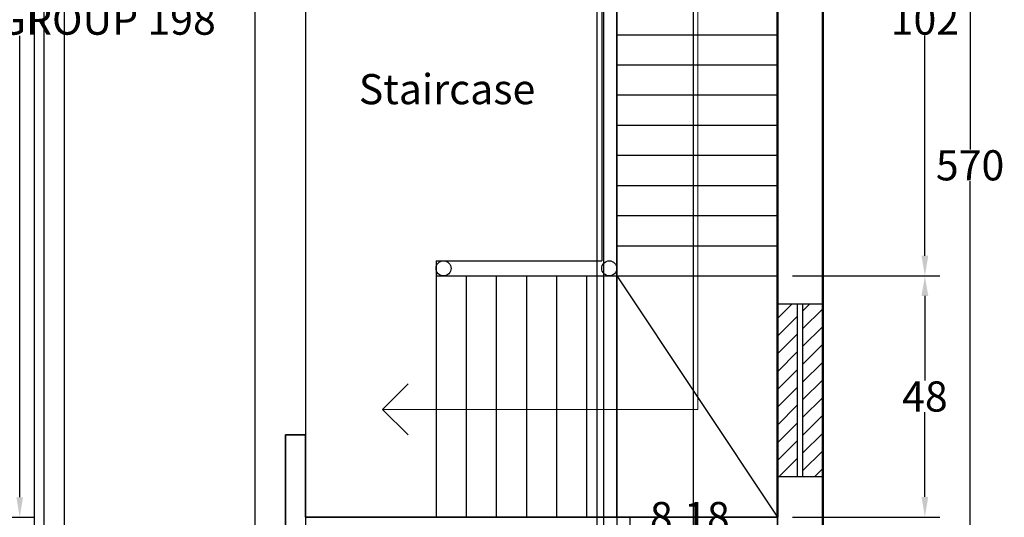
# Model space of a CAD drawing. Units: inches. Extents: x -1285 to -837, y -84 to 552.
# Tile 8 of 10: x -1037 to -841, y 164 to 263. Entities that reach past the tile are written whole.
import ezdxf

# ---------------------------------------------------------------- set-up
doc = ezdxf.new("R2010")
doc.units = ezdxf.units.IN
doc.header["$MEASUREMENT"] = 0
for name, color, linetype, lineweight in [('A-ANNO-DIMS', 2, 'Continuous', 18), ('A-ANNO-SYMB', 7, 'Continuous', 18), ('A-AREA-IDEN', 7, 'Continuous', 25), ('A-GLAZ-PATT', 191, 'Continuous', 13), ('Inner Wall', 202, 'Continuous', 35), ('Outer Wall', 12, 'Continuous', 50), ('Stairs', 90, 'Continuous', 25), ('Windows', 191, 'Continuous', 25)]:
    doc.layers.add(name, color=color, linetype=linetype, lineweight=lineweight)
doc.styles.get("Standard").update_dxf_attribs({"font": 'arial.ttf'})
doc.dimstyles.get("Standard").update_dxf_attribs({"dimtxt": 6, "dimasz": 4, "dimexe": 3, "dimexo": 3, "dimgap": 0.09, "dimtad": 0, "dimtih": 1, "dimtoh": 1, "dimdec": 1, "dimzin": 0, "dimdsep": 46, "dimlunit": 3, "dimtxsty": 'Standard', "dimcen": 0.09, "dimadec": 0, "dimazin": 0, "dimtfac": 1, "dimtdec": 1, "dimtofl": 0, "dimtmove": 0, "dimatfit": 3, "dimfxl": 1, "dimtolj": 1, "dimtzin": 0, "dimarcsym": 0})

# ---------------------------------------------------------------- blocks, each defined once
blk = doc.blocks.new('*D65')
at = {"layer": 'A-ANNO-DIMS', "color": 0, "lineweight": -2, "transparency": 16777216}
for p, q in [((-1064.13, 361.96), (-1034.42, 361.96)), ((-1037.42, 357.96), (-1037.42, 266.12)), ((-1037.42, 167.9), (-1037.42, 259.73)), ((-1064.13, 163.9), (-1034.42, 163.9))]:
    blk.add_line(p, q, dxfattribs=at)
at = {"layer": 'A-ANNO-DIMS', "color": 0, "transparency": 16777216}
for points in [[(-1038.09, 357.96), (-1036.75, 357.96), (-1037.42, 361.96)], [(-1038.09, 167.9), (-1036.75, 167.9), (-1037.42, 163.9)]]:
    blk.add_solid(points, dxfattribs=at)
at = {"layer": 'Defpoints', "color": 0, "transparency": 16777216}
for p in [(-1067.13, 361.96), (-1037.42, 361.96), (-1067.13, 163.9)]:
    blk.add_point(p, dxfattribs=at)
at = {"layer": 'A-ANNO-DIMS', "color": 0, "transparency": 16777216, "insert": (-1037.42, 262.93), "char_height": 6, "attachment_point": 5}
blk.add_mtext('\\A1;LOUNGE GROUP 198', dxfattribs=at)
blk = doc.blocks.new('*D70')
at = {"layer": 'A-ANNO-DIMS', "color": 0, "lineweight": -2, "transparency": 16777216}
for p, q in [((-874.53, 518.94), (-845.18, 518.94)), ((-848.18, 514.94), (-848.18, 237.09)), ((-848.18, -47.06), (-848.18, 230.79)), ((-874.53, -51.06), (-845.18, -51.06))]:
    blk.add_line(p, q, dxfattribs=at)
at = {"layer": 'A-ANNO-DIMS', "color": 0, "transparency": 16777216}
for points in [[(-848.85, 514.94), (-847.51, 514.94), (-848.18, 518.94)], [(-848.85, -47.06), (-847.51, -47.06), (-848.18, -51.06)]]:
    blk.add_solid(points, dxfattribs=at)
at = {"layer": 'Defpoints', "color": 0, "transparency": 16777216}
for p in [(-877.53, 518.94), (-848.18, 518.94), (-877.53, -51.06)]:
    blk.add_point(p, dxfattribs=at)
at = {"layer": 'A-ANNO-DIMS', "color": 0, "transparency": 16777216, "insert": (-848.18, 233.94), "char_height": 6, "attachment_point": 5}
blk.add_mtext('\\A1;570', dxfattribs=at)
blk = doc.blocks.new('*D80')
at = {"layer": 'A-ANNO-DIMS', "color": 0, "lineweight": -2, "transparency": 16777216}
for p, q in [((-1184.53, -13.66), (-1184.53, 551.29)), ((-1032.53, -13.66), (-1032.53, 551.29)), ((-1180.53, 548.29), (-1114.94, 548.29)), ((-1036.53, 548.29), (-1102.12, 548.29))]:
    blk.add_line(p, q, dxfattribs=at)
at = {"layer": 'A-ANNO-DIMS', "color": 0, "transparency": 16777216}
for points in [[(-1180.53, 548.96), (-1180.53, 547.62), (-1184.53, 548.29)], [(-1036.53, 548.96), (-1036.53, 547.62), (-1032.53, 548.29)]]:
    blk.add_solid(points, dxfattribs=at)
at = {"layer": 'Defpoints', "color": 0, "transparency": 16777216}
for p in [(-1032.53, 548.29), (-1184.53, -16.66), (-1032.53, -16.66)]:
    blk.add_point(p, dxfattribs=at)
at = {"layer": 'A-ANNO-DIMS', "color": 0, "transparency": 16777216, "insert": (-1108.53, 548.29), "char_height": 6, "attachment_point": 5}
blk.add_mtext('\\A1;152', dxfattribs=at)
blk = doc.blocks.new('*D85')
at = {"layer": 'A-ANNO-DIMS', "color": 0, "lineweight": -2, "transparency": 16777216}
for p, q in [((-980.53, 310.94), (-980.53, -83.53)), ((-922.53, 310.94), (-922.53, -83.53)), ((-976.53, -80.53), (-955.92, -80.53)), ((-926.53, -80.53), (-947.14, -80.53))]:
    blk.add_line(p, q, dxfattribs=at)
at = {"layer": 'A-ANNO-DIMS', "color": 0, "transparency": 16777216}
for points in [[(-976.53, -79.86), (-976.53, -81.2), (-980.53, -80.53)], [(-926.53, -79.86), (-926.53, -81.2), (-922.53, -80.53)]]:
    blk.add_solid(points, dxfattribs=at)
at = {"layer": 'Defpoints', "color": 0, "transparency": 16777216}
for p in [(-980.53, 313.94), (-922.53, 313.94), (-922.53, -80.53)]:
    blk.add_point(p, dxfattribs=at)
at = {"layer": 'A-ANNO-DIMS', "color": 0, "transparency": 16777216, "insert": (-951.53, -80.53), "char_height": 6, "attachment_point": 5}
blk.add_mtext('\\A1;58', dxfattribs=at)
blk = doc.blocks.new('*D86')
at = {"layer": 'A-ANNO-DIMS', "color": 0, "lineweight": -2, "transparency": 16777216}
for p, q in [((-918.53, 310.94), (-918.53, -83.53)), ((-886.53, 310.94), (-886.53, -83.53)), ((-914.53, -80.53), (-906.88, -80.53)), ((-890.53, -80.53), (-898.18, -80.53))]:
    blk.add_line(p, q, dxfattribs=at)
at = {"layer": 'A-ANNO-DIMS', "color": 0, "transparency": 16777216}
for points in [[(-914.53, -79.86), (-914.53, -81.2), (-918.53, -80.53)], [(-890.53, -79.86), (-890.53, -81.2), (-886.53, -80.53)]]:
    blk.add_solid(points, dxfattribs=at)
at = {"layer": 'Defpoints', "color": 0, "transparency": 16777216}
for p in [(-918.53, 313.94), (-886.53, 313.94), (-886.53, -80.53)]:
    blk.add_point(p, dxfattribs=at)
at = {"layer": 'A-ANNO-DIMS', "color": 0, "transparency": 16777216, "insert": (-902.53, -80.53), "char_height": 6, "attachment_point": 5}
blk.add_mtext('\\A1;32', dxfattribs=at)
blk = doc.blocks.new('*D93')
at = {"layer": 'A-ANNO-DIMS', "color": 0, "lineweight": -2, "transparency": 16777216}
for p, q in [((-1028.53, 78.94), (-1028.53, 551.29)), ((-990.53, 78.94), (-990.53, 551.29)), ((-1024.53, 548.29), (-1013.92, 548.29)), ((-994.53, 548.29), (-1005.14, 548.29))]:
    blk.add_line(p, q, dxfattribs=at)
at = {"layer": 'A-ANNO-DIMS', "color": 0, "transparency": 16777216}
for points in [[(-1024.53, 548.96), (-1024.53, 547.62), (-1028.53, 548.29)], [(-994.53, 548.96), (-994.53, 547.62), (-990.53, 548.29)]]:
    blk.add_solid(points, dxfattribs=at)
at = {"layer": 'Defpoints', "color": 0, "transparency": 16777216}
for p in [(-990.53, 548.29), (-1028.53, 75.94), (-990.53, 75.94)]:
    blk.add_point(p, dxfattribs=at)
at = {"layer": 'A-ANNO-DIMS', "color": 0, "transparency": 16777216, "insert": (-1009.53, 548.29), "char_height": 6, "attachment_point": 5}
blk.add_mtext('\\A1;38', dxfattribs=at)
blk = doc.blocks.new('*D94')
at = {"layer": 'A-ANNO-DIMS', "color": 0, "lineweight": -2, "transparency": 16777216}
for p, q in [((-883.53, 211.94), (-854.18, 211.94)), ((-857.18, 207.94), (-857.18, 191.09)), ((-857.18, 167.94), (-857.18, 184.79)), ((-883.53, 163.94), (-854.18, 163.94))]:
    blk.add_line(p, q, dxfattribs=at)
at = {"layer": 'A-ANNO-DIMS', "color": 0, "transparency": 16777216}
for points in [[(-857.85, 207.94), (-856.51, 207.94), (-857.18, 211.94)], [(-857.85, 167.94), (-856.51, 167.94), (-857.18, 163.94)]]:
    blk.add_solid(points, dxfattribs=at)
at = {"layer": 'Defpoints', "color": 0, "transparency": 16777216}
for p in [(-886.53, 211.94), (-886.53, 163.94), (-857.18, 163.94)]:
    blk.add_point(p, dxfattribs=at)
at = {"layer": 'A-ANNO-DIMS', "color": 0, "transparency": 16777216, "insert": (-857.18, 187.94), "char_height": 6, "attachment_point": 5}
blk.add_mtext('\\A1;48', dxfattribs=at)
blk = doc.blocks.new('*D95')
at = {"layer": 'A-ANNO-DIMS', "color": 0, "lineweight": -2, "transparency": 16777216}
for p, q in [((-883.53, 313.94), (-854.18, 313.94)), ((-857.18, 309.94), (-857.18, 266.09)), ((-857.18, 215.94), (-857.18, 259.79)), ((-883.53, 211.94), (-854.18, 211.94))]:
    blk.add_line(p, q, dxfattribs=at)
at = {"layer": 'A-ANNO-DIMS', "color": 0, "transparency": 16777216}
for points in [[(-857.85, 309.94), (-856.51, 309.94), (-857.18, 313.94)], [(-857.85, 215.94), (-856.51, 215.94), (-857.18, 211.94)]]:
    blk.add_solid(points, dxfattribs=at)
at = {"layer": 'Defpoints', "color": 0, "transparency": 16777216}
for p in [(-886.53, 313.94), (-886.53, 211.94), (-857.18, 211.94)]:
    blk.add_point(p, dxfattribs=at)
at = {"layer": 'A-ANNO-DIMS', "color": 0, "transparency": 16777216, "insert": (-857.18, 262.94), "char_height": 6, "attachment_point": 5}
blk.add_mtext('\\A1;102', dxfattribs=at)
blk = doc.blocks.new('*D97')
at = {"layer": 'A-ANNO-DIMS', "color": 0, "lineweight": -2, "transparency": 16777216}
for p, q in [((-921.19, 506.94), (-921.19, -83.53)), ((-886.53, 506.94), (-886.53, -83.53)), ((-917.19, -80.53), (-916.43, -80.53)), ((-890.53, -80.53), (-891.3, -80.53))]:
    blk.add_line(p, q, dxfattribs=at)
at = {"layer": 'A-ANNO-DIMS', "color": 0, "transparency": 16777216}
for points in [[(-917.19, -79.86), (-917.19, -81.2), (-921.19, -80.53)], [(-890.53, -79.86), (-890.53, -81.2), (-886.53, -80.53)]]:
    blk.add_solid(points, dxfattribs=at)
at = {"layer": 'Defpoints', "color": 0, "transparency": 16777216}
for p in [(-921.19, 509.94), (-886.53, 509.94), (-886.53, -80.53)]:
    blk.add_point(p, dxfattribs=at)
at = {"layer": 'A-ANNO-DIMS', "color": 0, "transparency": 16777216, "insert": (-903.86, -80.53), "char_height": 6, "attachment_point": 5}
blk.add_mtext('\\A1;34.665', dxfattribs=at)
blk = doc.blocks.new('*D102')
at = {"layer": 'A-ANNO-DIMS', "color": 0, "lineweight": -2, "transparency": 16777216}
for p, q in [((-903.24, -39.06), (-903.24, 551.29)), ((-886.53, -39.06), (-886.53, 551.29)), ((-899.24, 548.29), (-890.53, 548.29)), ((-886.53, 548.29), (-882.53, 548.29))]:
    blk.add_line(p, q, dxfattribs=at)
at = {"layer": 'A-ANNO-DIMS', "color": 0, "transparency": 16777216}
for points in [[(-899.24, 548.96), (-899.24, 547.62), (-903.24, 548.29)], [(-890.53, 548.96), (-890.53, 547.62), (-886.53, 548.29)]]:
    blk.add_solid(points, dxfattribs=at)
at = {"layer": 'Defpoints', "color": 0, "transparency": 16777216}
for p in [(-886.53, 548.29), (-903.24, -42.06), (-886.53, -42.06)]:
    blk.add_point(p, dxfattribs=at)
at = {"layer": 'A-ANNO-DIMS', "color": 0, "transparency": 16777216, "insert": (-873.18, 548.29), "char_height": 6, "attachment_point": 5}
blk.add_mtext('\\A1;16.71', dxfattribs=at)
blk = doc.blocks.new('*D104')
at = {"layer": 'A-ANNO-DIMS', "color": 0, "lineweight": -2, "transparency": 16777216}
for p, q in [((-1044.37, 506.94), (-1044.37, -83.53)), ((-1034.53, 506.94), (-1034.53, -83.53)), ((-1040.37, -80.53), (-1038.53, -80.53)), ((-1034.53, -80.53), (-1030.53, -80.53))]:
    blk.add_line(p, q, dxfattribs=at)
at = {"layer": 'A-ANNO-DIMS', "color": 0, "transparency": 16777216}
for points in [[(-1040.37, -79.86), (-1040.37, -81.2), (-1044.37, -80.53)], [(-1038.53, -79.86), (-1038.53, -81.2), (-1034.53, -80.53)]]:
    blk.add_solid(points, dxfattribs=at)
at = {"layer": 'Defpoints', "color": 0, "transparency": 16777216}
for p in [(-1044.37, 509.94), (-1034.53, 509.94), (-1034.53, -80.53)]:
    blk.add_point(p, dxfattribs=at)
at = {"layer": 'A-ANNO-DIMS', "color": 0, "transparency": 16777216, "insert": (-1022.66, -80.53), "char_height": 6, "attachment_point": 5}
blk.add_mtext('\\A1;9.84', dxfattribs=at)
blk = doc.blocks.new('*D114')
at = {"layer": 'A-ANNO-DIMS', "color": 0, "lineweight": -2, "transparency": 16777216}
for p, q in [((-915.88, 159.94), (-915.88, 163.94)), ((-915.88, 163.94), (-911.88, 163.94)), ((-889.53, 159.94), (-918.88, 159.94)), ((-915.88, 155.76), (-915.88, 155.94)), ((-889.53, 151.76), (-918.88, 151.76))]:
    blk.add_line(p, q, dxfattribs=at)
at = {"layer": 'A-ANNO-DIMS', "color": 0, "transparency": 16777216}
for points in [[(-916.55, 155.94), (-915.21, 155.94), (-915.88, 159.94)], [(-916.55, 155.76), (-915.21, 155.76), (-915.88, 151.76)]]:
    blk.add_solid(points, dxfattribs=at)
at = {"layer": 'Defpoints', "color": 0, "transparency": 16777216}
for p in [(-915.88, 159.94), (-886.53, 159.94), (-886.53, 151.76)]:
    blk.add_point(p, dxfattribs=at)
at = {"layer": 'A-ANNO-DIMS', "color": 0, "transparency": 16777216, "insert": (-903.99, 163.94), "char_height": 6, "attachment_point": 5}
blk.add_mtext('\\A1;8.18', dxfattribs=at)

msp = doc.modelspace()

# ---------------------------------------------------------------- hatches: boundary and pattern name
at = {"layer": 'A-GLAZ-PATT'}
h = msp.add_hatch(dxfattribs=at)
h.set_pattern_fill('ANSI31', color=256, scale=20)
h.set_pattern_definition([(45, (-2191.666, -702.1458), (-1.767767, 1.767767), [])])
h.paths.add_polyline_path([(-877.5299, 206.2979), (-881.5299, 206.2979), (-881.5299, 171.9493), (-877.5299, 171.9493)])
h.paths.add_polyline_path([(-882.5299, 206.2979), (-886.5299, 206.2979), (-886.5299, 171.9493), (-882.5299, 171.9493)])

# ---------------------------------------------------------------- linework, layer by layer
at = {"layer": 'A-ANNO-SYMB'}
for p, q in [((-902.4002, 338.1338), (-902.4002, 185.376)), ((-965.1755, 185.376), (-960.0865, 190.4519)), ((-902.4002, 185.376), (-965.1755, 185.376)), ((-965.1755, 185.376), (-960.0865, 180.3001))]:
    msp.add_line(p, q, dxfattribs=at)
at = {"layer": 'Inner Wall'}
for p, q in [((-918.5299, 361.9392), (-918.5299, 211.9392)), ((-980.5299, 180.3238), (-984.5299, 180.3238)), ((-984.5299, 180.3238), (-984.5299, 75.9392)), ((-980.5299, 180.3238), (-980.5299, 163.9392)), ((-980.5299, 163.9392), (-886.5299, 163.9392))]:
    msp.add_line(p, q, dxfattribs=at)
at = {"layer": 'Outer Wall'}
for p, q in [((-877.5299, 518.9392), (-877.5299, -51.0608)), ((-886.5299, 361.9392), (-886.5299, 163.9392))]:
    msp.add_line(p, q, dxfattribs=at)
at = {"layer": 'Stairs'}
for p, q in [((-921.5299, 309.9392), (-921.5299, 214.9392)), ((-918.5299, 259.9392), (-886.5299, 259.9392)), ((-918.5299, 253.9392), (-886.5299, 253.9392)), ((-918.5299, 247.9392), (-886.5299, 247.9392)), ((-918.5299, 241.9392), (-886.5299, 241.9392)), ((-918.5299, 235.9392), (-886.5299, 235.9392)), ((-918.5299, 229.9392), (-886.5299, 229.9392)), ((-918.5299, 223.9392), (-886.5299, 223.9392)), ((-918.5299, 217.9392), (-886.5299, 217.9392)), ((-954.5299, 214.9392), (-954.5299, 163.9392)), ((-954.5299, 214.9392), (-921.5299, 214.9392)), ((-954.5299, 211.9392), (-918.5299, 211.9392)), ((-948.5299, 211.9392), (-948.5299, 163.9392)), ((-942.5299, 211.9392), (-942.5299, 163.9392)), ((-936.5299, 211.9392), (-936.5299, 163.9392)), ((-930.5299, 211.9392), (-930.5299, 163.9392)), ((-924.5299, 211.9392), (-924.5299, 163.9392)), ((-918.5299, 163.9392), (-918.5299, 211.9392)), ((-918.5299, 211.9392), (-886.5299, 211.9392)), ((-918.5299, 211.9392), (-886.5299, 163.9392))]:
    msp.add_line(p, q, dxfattribs=at)
for centre in [(-953.0299, 213.4392), (-920.0299, 213.4392)]:
    msp.add_circle(centre, 1.5, dxfattribs=at)
at = {"layer": 'Windows'}
for p, q in [((-877.5299, 206.2979), (-886.5299, 206.2979)), ((-882.5299, 171.9493), (-882.5299, 206.2979)), ((-881.5299, 206.2979), (-881.5299, 171.9493))]:
    msp.add_line(p, q, dxfattribs=at)
msp.add_lwpolyline([(-877.5299, 206.2979), (-877.5299, 171.9493), (-886.5299, 171.9493), (-886.5299, 206.2979)], dxfattribs=at)

# ---------------------------------------------------------------- texts
at = {"layer": 'A-AREA-IDEN', "insert": (-986.722, 252.1011), "char_height": 6, "attachment_point": 1}
msp.add_mtext_dynamic_manual_height_columns('\\pxqc;Staircase', width=68.784729, gutter_width=1, heights=[0], dxfattribs=at)

# ---------------------------------------------------------------- dimensions: what is measured, and where the dimension line sits
at = {"layer": 'A-ANNO-DIMS'}
for base, p1, p2, override, picture, middle in [((-1032.5299, 548.2892), (-1184.5299, -16.6608), (-1032.5299, -16.6608), {"dimdec": 0, "dimlfac": 1, "dimrnd": 0, "dimzin": 0, "dimdsep": 46, "dimlunit": 2}, '*D80', (-1108.5299, 548.2892)), ((-990.5299, 548.2892), (-1028.5299, 75.9392), (-990.5299, 75.9392), {"dimdec": 0, "dimlfac": 1, "dimrnd": 0, "dimzin": 0, "dimdsep": 46, "dimlunit": 2}, '*D93', (-1009.5299, 548.2892)), ((-886.5299, 548.2892), (-903.24, -42.0608), (-886.5299, -42.0608), {"dimdec": 2, "dimlfac": 1, "dimrnd": 0, "dimzin": 0, "dimdsep": 46, "dimlunit": 2}, '*D102', (-873.1779, 548.2892)), ((-1034.5299, -80.5308), (-1044.3703, 509.9392), (-1034.5299, 509.9392), {"dimdec": 2, "dimlfac": 1, "dimrnd": 0, "dimzin": 0, "dimdsep": 46, "dimlunit": 2}, '*D104', (-1022.6595, -80.5308)), ((-886.5299, -80.5308), (-921.1945, 509.9392), (-886.5299, 509.9392), {"dimdec": 3, "dimlfac": 1, "dimrnd": 0, "dimzin": 0, "dimdsep": 46, "dimlunit": 2}, '*D97', (-903.8622, -80.5308)), ((-922.5299, -80.5308), (-980.5299, 313.9392), (-922.5299, 313.9392), {"dimdec": 0, "dimlfac": 1, "dimrnd": 0, "dimzin": 0, "dimdsep": 46, "dimlunit": 2}, '*D85', (-951.5299, -80.5308)), ((-886.5299, -80.5308), (-918.5299, 313.9392), (-886.5299, 313.9392), {"dimdec": 0, "dimlfac": 1, "dimrnd": 0, "dimzin": 0, "dimdsep": 46, "dimlunit": 2}, '*D86', (-902.5299, -80.5308))]:
    dim = msp.add_linear_dim(base=base, p1=p1, p2=p2, dimstyle='Standard', override=override, dxfattribs=at)
    dim.commit()
    dim.dimension.update_dxf_attribs({"geometry": picture, "text_midpoint": middle})
for base, p1, p2, angle, override, picture, middle in [((-848.1799, 518.9392), (-877.5299, -51.0608), (-877.5299, 518.9392), 90, {"dimdec": 0, "dimlfac": 1, "dimrnd": 0, "dimzin": 0, "dimdsep": 46, "dimlunit": 2}, '*D70', (-848.1799, 233.9392)), ((-857.1799, 211.9392), (-886.5299, 313.9392), (-886.5299, 211.9392), 270, {"dimdec": 0, "dimlfac": 1, "dimrnd": 0, "dimzin": 0, "dimdsep": 46, "dimlunit": 2}, '*D95', (-857.1799, 262.9392)), ((-857.1799, 163.9392), (-886.5299, 211.9392), (-886.5299, 163.9392), 270, {"dimdec": 0, "dimlfac": 1, "dimrnd": 0, "dimzin": 0, "dimdsep": 46, "dimlunit": 2}, '*D94', (-857.1799, 187.9392)), ((-915.8799, 159.9392), (-886.5299, 151.7586), (-886.5299, 159.9392), 90, {"dimdec": 2, "dimlfac": 1, "dimrnd": 0, "dimzin": 0, "dimdsep": 46, "dimlunit": 2}, '*D114', (-903.987, 163.9392))]:
    dim = msp.add_linear_dim(base=base, p1=p1, p2=p2, angle=angle, dimstyle='Standard', override=override, dxfattribs=at)
    dim.commit()
    dim.dimension.update_dxf_attribs({"geometry": picture, "text_midpoint": middle})
dim = msp.add_linear_dim(base=(-1037.4189, 361.9592), p1=(-1067.1282, 163.8976), p2=(-1067.1282, 361.9592), angle=90, text='LOUNGE GROUP <>', dimstyle='Standard', override={"dimdec": 0, "dimlfac": 1, "dimrnd": 0, "dimzin": 0, "dimdsep": 46, "dimlunit": 2}, dxfattribs=at)
dim.commit()
dim.dimension.update_dxf_attribs({"geometry": '*D65', "text_midpoint": (-1037.4189, 262.9284)})

doc.saveas('drawing.dxf')
